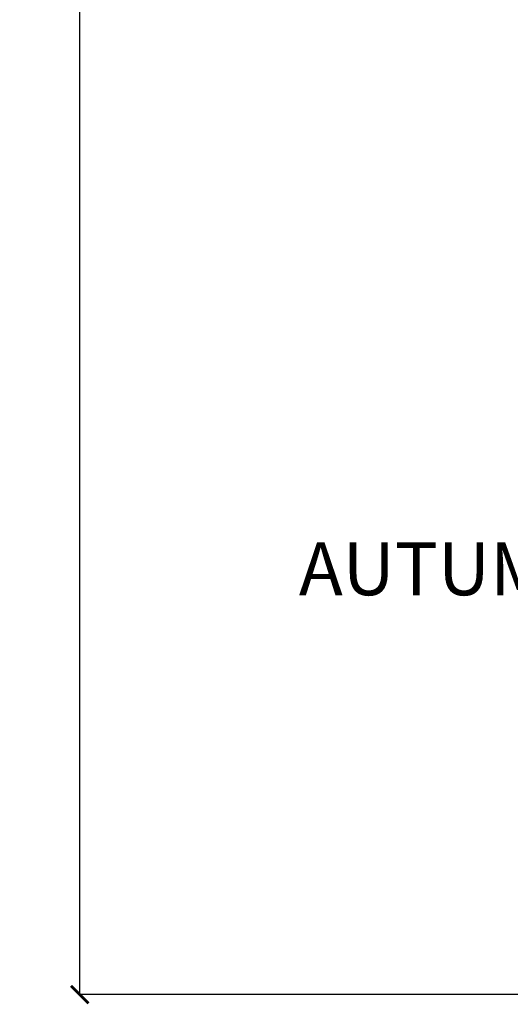
# Model space of a CAD drawing. Units: inches. Extents: x 1704 to 6393, y -157 to 1172.
# Tile 9 of 122: x 1823 to 1879, y 89 to 201. Entities that reach past the tile are written whole.
import ezdxf

# ---------------------------------------------------------------- set-up
doc = ezdxf.new("R2010")
doc.units = ezdxf.units.IN
doc.header["$MEASUREMENT"] = 0
doc.layers.add('A-ANNO-DIMS', color=7, linetype='Continuous', lineweight=13)
doc.styles.get("Standard").update_dxf_attribs({"font": 'arial.ttf'})
doc.dimstyles.get("Standard").update_dxf_attribs({"dimtxt": 6, "dimasz": 2, "dimexe": 0.18, "dimexo": 0.0625, "dimgap": 0.09, "dimtad": 0, "dimtih": 1, "dimtoh": 1, "dimdec": 1, "dimzin": 0, "dimdsep": 46, "dimlunit": 3, "dimtxsty": 'Standard', "dimblk": 'ARCHTICK', "dimcen": 0.09, "dimadec": 0, "dimazin": 0, "dimtfac": 1, "dimtdec": 1, "dimtofl": 0, "dimtmove": 0, "dimatfit": 3, "dimfxl": 1, "dimtolj": 1, "dimtzin": 0, "dimarcsym": 0})

# ---------------------------------------------------------------- blocks, each defined once
blk = doc.blocks.new('_ArchTick')
at = {"color": 0, "linetype": 'ByBlock', "const_width": 0.15}
blk.add_lwpolyline([(-0.5, -0.5), (0.5, 0.5)], dxfattribs=at)
blk = doc.blocks.new('*D78')
at = {"layer": 'A-ANNO-DIMS', "color": 0, "lineweight": -2, "transparency": 16777216}
for p, q in [((1896.87, 155.25), (1891.74, 155.25)), ((1891.92, 155.25), (1891.92, 141.74)), ((1891.92, 121.85), (1891.92, 135.35)), ((1896.87, 121.85), (1891.74, 121.85))]:
    blk.add_line(p, q, dxfattribs=at)
at = {"layer": 'Defpoints', "color": 0, "lineweight": -3, "transparency": 16777216}
for p in [(1896.93, 155.25), (1891.92, 121.85), (1896.93, 121.85)]:
    blk.add_point(p, dxfattribs=at)
at = {"layer": 'A-ANNO-DIMS', "color": 0, "lineweight": -2, "transparency": 16777216, "xscale": 2, "yscale": 2, "zscale": 2}
for p, rotation in [((1891.92, 155.25), 90), ((1891.92, 121.85), 270)]:
    blk.add_blockref('_ArchTick', p, dxfattribs=dict(at, rotation=rotation))
at = {"layer": 'A-ANNO-DIMS', "color": 0, "transparency": 16777216, "insert": (1891.92, 138.55), "char_height": 6, "attachment_point": 5}
blk.add_mtext('\\A1;AUTUMN SHRUB 33', dxfattribs=at)
blk = doc.blocks.new('*D93')
at = {"layer": 'A-ANNO-DIMS', "color": 0, "lineweight": -2, "transparency": 16777216}
for p, q in [((2605.29, 895.21), (1829.7, 895.21)), ((1829.88, 895.21), (1829.88, 495.87)), ((1829.88, 90.21), (1829.88, 489.56)), ((2605.29, 90.21), (1829.7, 90.21))]:
    blk.add_line(p, q, dxfattribs=at)
at = {"layer": 'Defpoints', "color": 0, "lineweight": -3, "transparency": 16777216}
for p in [(2605.35, 895.21), (1829.88, 90.21), (2605.35, 90.21)]:
    blk.add_point(p, dxfattribs=at)
at = {"layer": 'A-ANNO-DIMS', "color": 0, "lineweight": -2, "transparency": 16777216, "xscale": 2, "yscale": 2, "zscale": 2}
for p, rotation in [((1829.88, 895.21), 90), ((1829.88, 90.21), 270)]:
    blk.add_blockref('_ArchTick', p, dxfattribs=dict(at, rotation=rotation))
at = {"layer": 'A-ANNO-DIMS', "color": 0, "transparency": 16777216, "insert": (1829.88, 492.71), "char_height": 6, "attachment_point": 5}
blk.add_mtext('\\A1;805', dxfattribs=at)

msp = doc.modelspace()

# ---------------------------------------------------------------- dimensions: what is measured, and where the dimension line sits
at = {"layer": 'A-ANNO-DIMS'}
dim = msp.add_linear_dim(base=(1829.878, 90.213), p1=(2605.349, 895.213), p2=(2605.349, 90.213), angle=90, dimstyle='Standard', override={"dimdec": 0, "dimlfac": 1, "dimrnd": 0, "dimzin": 0, "dimdsep": 46, "dimlunit": 2}, dxfattribs=at)
dim.commit()
dim.dimension.update_dxf_attribs({"geometry": '*D93', "text_midpoint": (1829.878, 492.713)})
dim = msp.add_linear_dim(base=(1891.923, 121.849), p1=(1896.932, 155.246), p2=(1896.932, 121.849), angle=270, text='AUTUMN SHRUB <>', dimstyle='Standard', override={"dimdec": 0, "dimlfac": 1, "dimrnd": 0, "dimzin": 0, "dimdsep": 46, "dimlunit": 2}, dxfattribs=at)
dim.commit()
dim.dimension.update_dxf_attribs({"geometry": '*D78', "text_midpoint": (1891.923, 138.547)})

doc.saveas('drawing.dxf')
